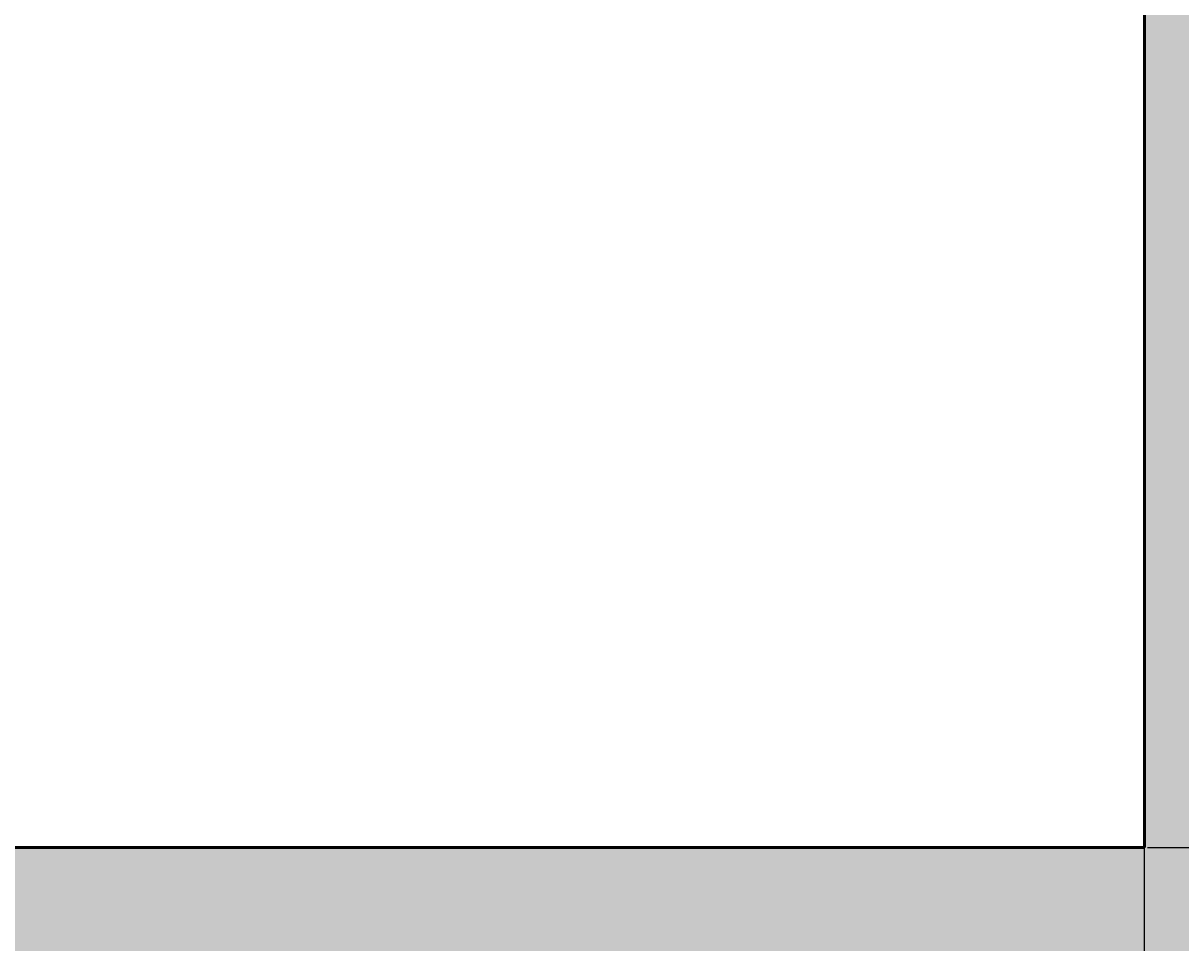
# Model space of a CAD drawing. Units: inches. Extents: x 2231 to 2461, y 2045 to 2455.
# Tile 82 of 95: x 2409 to 2434, y 2333 to 2352. Entities that reach past the tile are written whole.
import ezdxf

# ---------------------------------------------------------------- set-up
doc = ezdxf.new("R2010")
doc.units = ezdxf.units.IN
doc.layers.add('A-ANNO-DIMS', color=2, linetype='Continuous', lineweight=18)
doc.layers.add('A-WALL', color=7, linetype='Continuous', lineweight=50)
doc.layers.add('A-WALL-PATT', color=18, linetype='Continuous', lineweight=13, true_color=0x000000)
doc.styles.get("Standard").update_dxf_attribs({"font": 'arial.ttf'})
doc.dimstyles.get("Standard").update_dxf_attribs({"dimtxt": 0.18, "dimasz": 0.18, "dimexe": 0.18, "dimexo": 0.0625, "dimgap": 0.09, "dimtad": 0, "dimtih": 1, "dimtoh": 1, "dimdec": 4, "dimzin": 0, "dimdsep": 46, "dimtxsty": 'Standard', "dimcen": 0.09, "dimadec": 0, "dimazin": 0, "dimtfac": 1, "dimtdec": 4, "dimtofl": 0, "dimtmove": 0, "dimatfit": 3, "dimfxl": 1, "dimtolj": 1, "dimtzin": 0, "dimarcsym": 0})

# ---------------------------------------------------------------- blocks, each defined once
blk = doc.blocks.new('*D38')
at = {"layer": 'A-ANNO-DIMS', "color": 0, "lineweight": -2, "transparency": 16777216}
for p, q in [((2432.856, 2426.833), (2460.606, 2426.833)), ((2460.426, 2426.653), (2460.426, 2381.015)), ((2460.426, 2335.013), (2460.426, 2380.651)), ((2432.856, 2334.833), (2460.606, 2334.833))]:
    blk.add_line(p, q, dxfattribs=at)
at = {"layer": 'A-ANNO-DIMS', "color": 0, "transparency": 16777216}
for points in [[(2460.396, 2426.653), (2460.456, 2426.653), (2460.426, 2426.833)], [(2460.396, 2335.013), (2460.456, 2335.013), (2460.426, 2334.833)]]:
    blk.add_solid(points, dxfattribs=at)
at = {"layer": 'Defpoints', "color": 0, "transparency": 16777216}
for p in [(2432.794, 2426.833), (2460.426, 2426.833), (2432.794, 2334.833)]:
    blk.add_point(p, dxfattribs=at)
at = {"layer": 'A-ANNO-DIMS', "color": 0, "transparency": 16777216, "insert": (2460.426, 2380.833), "char_height": 0.18, "attachment_point": 5}
blk.add_mtext('\\A1;92', dxfattribs=at)
blk = doc.blocks.new('*D42')
at = {"layer": 'A-ANNO-DIMS', "color": 0, "lineweight": -2, "transparency": 16777216}
for p, q in [((2396.794, 2286.895), (2396.794, 2454.645)), ((2432.794, 2286.895), (2432.794, 2454.645)), ((2396.974, 2454.465), (2414.575, 2454.465)), ((2432.614, 2454.465), (2415.012, 2454.465))]:
    blk.add_line(p, q, dxfattribs=at)
at = {"layer": 'A-ANNO-DIMS', "color": 0, "transparency": 16777216}
for points in [[(2396.974, 2454.495), (2396.974, 2454.435), (2396.794, 2454.465)], [(2432.614, 2454.495), (2432.614, 2454.435), (2432.794, 2454.465)]]:
    blk.add_solid(points, dxfattribs=at)
at = {"layer": 'Defpoints', "color": 0, "transparency": 16777216}
for p in [(2432.794, 2454.465), (2396.794, 2286.833), (2432.794, 2286.833)]:
    blk.add_point(p, dxfattribs=at)
at = {"layer": 'A-ANNO-DIMS', "color": 0, "transparency": 16777216, "insert": (2414.794, 2454.465), "char_height": 0.18, "attachment_point": 5}
blk.add_mtext('\\A1;36', dxfattribs=at)
blk = doc.blocks.new('*D59')
at = {"layer": 'A-ANNO-DIMS', "color": 0, "lineweight": -2, "transparency": 16777216}
for p, q in [((2408.794, 2182.895), (2408.794, 2454.645)), ((2432.794, 2182.895), (2432.794, 2454.645)), ((2408.974, 2454.465), (2420.573, 2454.465)), ((2432.614, 2454.465), (2421.014, 2454.465))]:
    blk.add_line(p, q, dxfattribs=at)
at = {"layer": 'A-ANNO-DIMS', "color": 0, "transparency": 16777216}
for points in [[(2408.974, 2454.495), (2408.974, 2454.435), (2408.794, 2454.465)], [(2432.614, 2454.495), (2432.614, 2454.435), (2432.794, 2454.465)]]:
    blk.add_solid(points, dxfattribs=at)
at = {"layer": 'Defpoints', "color": 0, "transparency": 16777216}
for p in [(2432.794, 2454.465), (2408.794, 2182.833), (2432.794, 2182.833)]:
    blk.add_point(p, dxfattribs=at)
at = {"layer": 'A-ANNO-DIMS', "color": 0, "transparency": 16777216, "insert": (2420.794, 2454.465), "char_height": 0.18, "attachment_point": 5}
blk.add_mtext('\\A1;24', dxfattribs=at)
blk = doc.blocks.new('*D76')
at = {"layer": 'A-ANNO-DIMS', "color": 0, "lineweight": -2, "transparency": 16777216}
for p, q in [((2422.106, 2352.663), (2460.606, 2352.663)), ((2460.426, 2352.483), (2460.426, 2343.93)), ((2460.426, 2335.013), (2460.426, 2343.566)), ((2432.856, 2334.833), (2460.606, 2334.833))]:
    blk.add_line(p, q, dxfattribs=at)
at = {"layer": 'A-ANNO-DIMS', "color": 0, "transparency": 16777216}
for points in [[(2460.396, 2352.483), (2460.456, 2352.483), (2460.426, 2352.663)], [(2460.396, 2335.013), (2460.456, 2335.013), (2460.426, 2334.833)]]:
    blk.add_solid(points, dxfattribs=at)
at = {"layer": 'Defpoints', "color": 0, "transparency": 16777216}
for p in [(2422.043, 2352.663), (2460.426, 2352.663), (2432.794, 2334.833)]:
    blk.add_point(p, dxfattribs=at)
at = {"layer": 'A-ANNO-DIMS', "color": 0, "transparency": 16777216, "insert": (2460.426, 2343.748), "char_height": 0.18, "attachment_point": 5}
blk.add_mtext('\\A1;17.83', dxfattribs=at)

msp = doc.modelspace()

# ---------------------------------------------------------------- hatches: boundary and pattern name
at = {"layer": 'A-WALL-PATT'}
h = msp.add_hatch(color=256, dxfattribs=at)
h.dxf.hatch_style = 1
h.paths.add_polyline_path([(2441.7935, 2269.1535), (2432.7935, 2269.1535), (2432.7935, 2186.8328), (2396.7935, 2186.8328), (2396.7935, 2286.8328), (2394.7935, 2286.8328), (2394.7935, 2186.8328), (2334.7935, 2186.8328), (2334.7935, 2182.8328), (2432.7935, 2182.8328), (2432.7935, 2072.8328), (2416.6639, 2072.8328), (2416.6639, 2063.8328), (2441.7935, 2063.8328)])
h.paths.add_polyline_path([(2368.6639, 2072.8328), (2367.04, 2072.8328), (2330.7942, 2072.8328), (2330.7397, 2063.8328), (2368.6639, 2063.8328)])
h.paths.add_polyline_path([(2300.7392, 2068.3328), (2300.7392, 2072.8328), (2298.7935, 2072.8328), (2294.7935, 2072.8328), (2258.7935, 2072.8328), (2258.7935, 2120.8328), (2294.7935, 2120.8328), (2298.7935, 2120.8328), (2298.7935, 2128.8328), (2294.7935, 2128.8328), (2294.7935, 2124.8328), (2258.7935, 2124.8328), (2258.7935, 2182.8328), (2294.7935, 2182.8328), (2294.7935, 2174.8328), (2298.7935, 2174.8328), (2298.7935, 2182.8328), (2304.7935, 2182.8328), (2304.7935, 2186.8328), (2258.7935, 2186.8328), (2258.7935, 2221.999), (2249.7935, 2221.999), (2249.7935, 2063.8328), (2300.7392, 2063.8328)])
h.paths.add_polyline_path([(2391.9338, 2435.8328), (2333.82, 2435.8328), (2333.82, 2426.8328), (2368.7935, 2426.8328), (2368.7935, 2374.9508), (2368.7935, 2370.8328), (2372.3935, 2370.8328), (2372.7935, 2370.8328), (2372.7935, 2426.8328), (2391.9338, 2426.8328)])
h.paths.add_polyline_path([(2441.7935, 2435.8328), (2415.9338, 2435.8328), (2415.9338, 2426.8328), (2432.7935, 2426.8328), (2432.7935, 2334.8328), (2372.7935, 2334.8328), (2372.7935, 2346.8328), (2368.7935, 2346.8328), (2368.7935, 2306.8328), (2360.7935, 2306.8328), (2360.7935, 2302.8328), (2368.7935, 2302.8328), (2372.7935, 2302.8328), (2372.7935, 2330.8328), (2432.7935, 2330.8328), (2432.7935, 2317.1535), (2441.7935, 2317.1535)])
h.paths.add_polyline_path([(2285.82, 2435.8328), (2249.7935, 2435.8328), (2249.7935, 2269.999), (2258.7935, 2269.999), (2258.7935, 2302.8328), (2318.8168, 2302.8328), (2330.7935, 2302.8328), (2330.7935, 2306.8328), (2258.7935, 2306.8328), (2258.7935, 2426.8328), (2285.82, 2426.8328)])

# ---------------------------------------------------------------- linework, layer by layer
at = {"layer": 'A-WALL'}
for p in [(2432.7935, 2426.8328), (2372.7935, 2334.8328)]:
    msp.add_line(p, (2432.7935, 2334.8328), dxfattribs=at)

# ---------------------------------------------------------------- dimensions: what is measured, and where the dimension line sits
at = {"layer": 'A-ANNO-DIMS'}
for p1, p2, picture, middle in [((2396.7935, 2286.8328), (2432.7935, 2286.8328), '*D42', (2414.7935, 2454.4653)), ((2408.7935, 2182.8328), (2432.7935, 2182.8328), '*D59', (2420.7935, 2454.4653))]:
    dim = msp.add_linear_dim(base=(2432.7935, 2454.4653), p1=p1, p2=p2, dimstyle='Standard', override={"dimdec": 0, "dimlfac": 1, "dimrnd": 0, "dimzin": 0, "dimdsep": 46, "dimlunit": 2}, dxfattribs=at)
    dim.commit()
    dim.dimension.update_dxf_attribs({"geometry": picture, "text_midpoint": middle})
for base, p2, override, picture, middle in [((2460.426, 2426.8328), (2432.7935, 2426.8328), {"dimdec": 0, "dimlfac": 1, "dimrnd": 0, "dimzin": 0, "dimdsep": 46, "dimlunit": 2}, '*D38', (2460.426, 2380.8328)), ((2460.426, 2352.6633), (2422.0433, 2352.6633), {"dimdec": 2, "dimlfac": 1, "dimrnd": 0, "dimzin": 0, "dimdsep": 46, "dimlunit": 2}, '*D76', (2460.426, 2343.7481))]:
    dim = msp.add_linear_dim(base=base, p1=(2432.7935, 2334.8328), p2=p2, angle=90, dimstyle='Standard', override=override, dxfattribs=at)
    dim.commit()
    dim.dimension.update_dxf_attribs({"geometry": picture, "text_midpoint": middle})

doc.saveas('drawing.dxf')
